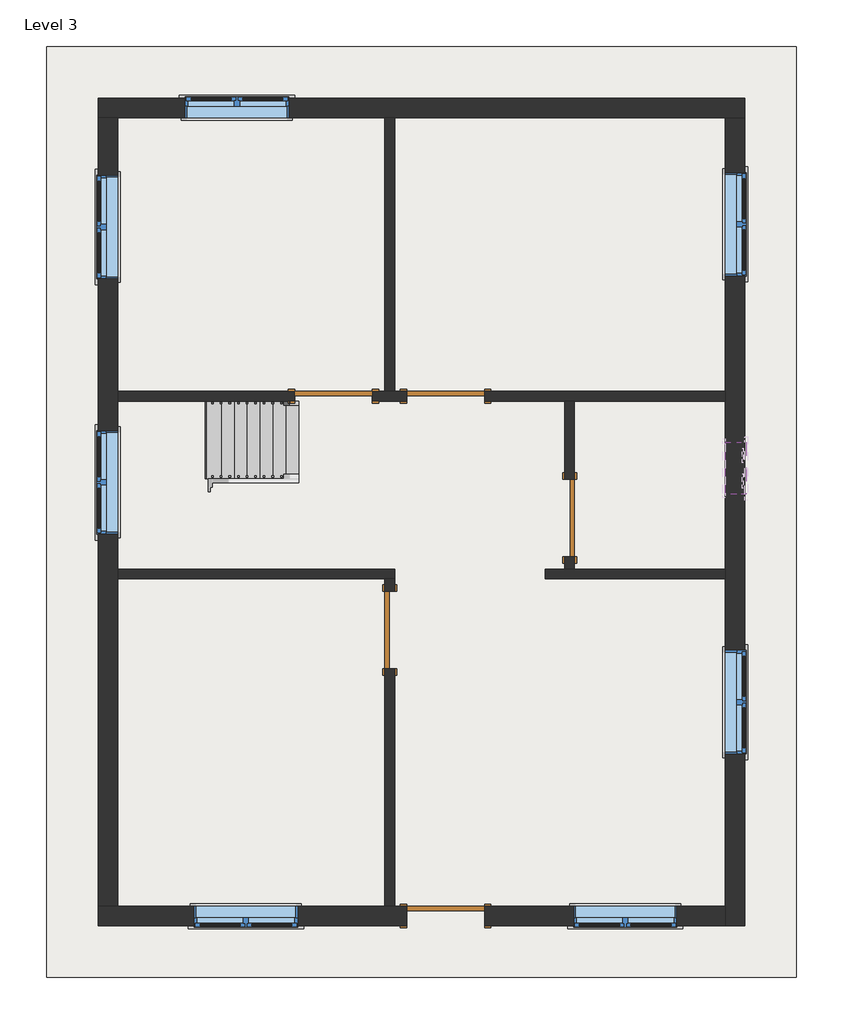
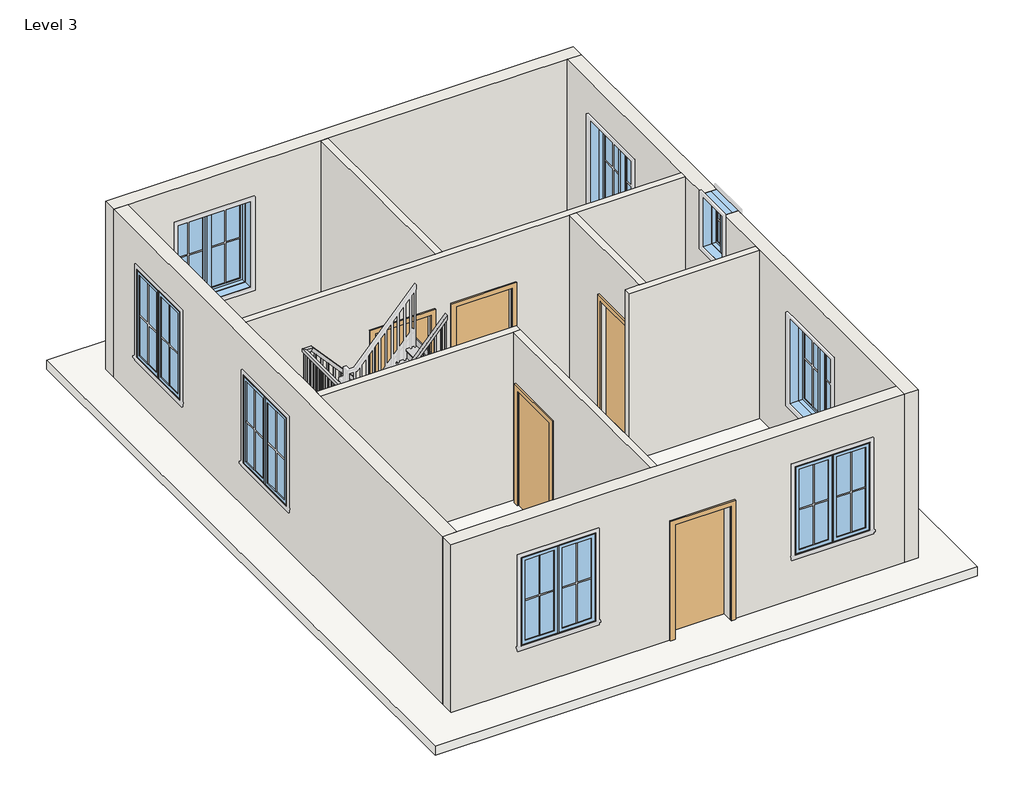
# One storey, part 1 of 2: 10 walls, 8 windows, 5 doors, 1 railing, 1 roof, 1 stair flight.
"""IFC4 building model written with IfcOpenShell, lengths in millimetres."""

from ifc_helpers import new_model, si_unit, frame, origin, place, context, project, spatial, polyline, outline, extrude, faceted_brep, transform, mapped, element, save
from components import door_e5f9f3c4, door_305aa2a5, door_a90ba1ad, stair_flight_173d3475, window_c417fced, window_8377141f

model = new_model("IFC4")

# Units and contexts
model_context = context("Model", 3, world=origin())
ifc_project = project(units=[si_unit("LENGTHUNIT", "METRE", prefix="MILLI")], contexts=[model_context])

# Site, building, storey
site = spatial("IfcSite", under=ifc_project)
building = spatial("IfcBuilding", under=site)
storey = spatial("IfcBuildingStorey", under=building, Name="Level 3", Elevation=6096.0)

# Doors
placement = place(None, origin())
door_shape = door_e5f9f3c4(model_context)
element("IfcDoor", 1, ObjectType="Single-Flush : 36\" x 84\"", at=placement, inside=storey, context=model_context, shape_type="MappedRepresentation", body=[
    mapped(door_shape, transform((4044.95, 10966.45, 6096.0), x_axis=(1.0, 0.0, 0.0), y_axis=(0.0, 1.0, 0.0), z_axis=(0.0, 0.0, 1.0))),
])
element("IfcDoor", 2, ObjectType="Single-Flush : 36\" x 84\"", at=placement, inside=storey, context=model_context, shape_type="MappedRepresentation", body=[
    mapped(door_shape, transform((4705.35, 8210.55, 6096.0), x_axis=(0.0, 1.0, 0.0), y_axis=(-1.0, 0.0, 0.0), z_axis=(0.0, 0.0, 1.0))),
])
element("IfcDoor", 3, ObjectType="Single-Flush : 36\" x 84\"", at=placement, inside=storey, context=model_context, shape_type="MappedRepresentation", body=[
    mapped(door_shape, transform((6826.25, 9531.35, 6096.0), x_axis=(0.0, -1.0, 0.0), y_axis=(1.0, 0.0, 0.0), z_axis=(0.0, 0.0, 1.0))),
])
door_2_shape = door_305aa2a5(model_context)
element("IfcDoor", 4, ObjectType="Single-Flush : 36\" x 84\"", at=placement, inside=storey, context=model_context, shape_type="MappedRepresentation", body=[
    mapped(door_2_shape, transform((5365.75, 10966.45, 6096.0), x_axis=(-1.0, 0.0, 0.0), y_axis=(0.0, -1.0, 0.0), z_axis=(0.0, 0.0, 1.0))),
])
door_3_shape = door_a90ba1ad(model_context)
element("IfcDoor", 5, ObjectType="Single-Flush : 36\" x 84\"", at=placement, inside=storey, context=model_context, shape_type="MappedRepresentation", body=[
    mapped(door_3_shape, transform((5365.75, 4838.7, 6096.0), x_axis=(-1.0, 0.0, 0.0), y_axis=(0.0, -1.0, 0.0), z_axis=(0.0, 0.0, 1.0))),
])

# Railing
element("IfcRailing", 6, ObjectType="Handrail - Rectangular", at=placement, inside=storey, context=model_context, shape_type="SolidModel", body=[
    faceted_brep([(3632.2, 10858.5, 7179.7333333), (3632.2, 10858.5, 7103.7950998), (3632.2, 10909.3, 7103.7950998), (3632.2, 10909.3, 7179.7333333), (2565.4, 10858.5, 8365.0666667), (2542.7755898, 10858.5, 8314.2666667), (2542.7755898, 10909.3, 8314.2666667), (2565.4, 10909.3, 8365.0666667), (2463.8, 10858.5, 8365.0666667), (2463.8, 10858.5, 8314.2666667), (2413.0, 10909.3, 8314.2666667), (2413.0, 10909.3, 8365.0666667), (2463.8, 9055.1, 8365.0666667), (2463.8, 9004.3, 8314.2666667), (2413.0, 9004.3, 8314.2666667), (2413.0, 9055.1, 8365.0666667), (2463.8, 9055.1, 8506.1777778), (2463.8, 9004.3, 8455.3777778), (2413.0, 9004.3, 8455.3777778), (2413.0, 9055.1, 8506.1777778), (2463.8, 8978.9, 8506.1777778), (2463.8, 8978.9, 8455.3777778), (2413.0, 8928.1, 8455.3777778), (2413.0, 8928.1, 8506.1777778), (2540.0, 8978.9, 8506.1777778), (2562.6244102, 8978.9, 8455.3777778), (2562.6244102, 8928.1, 8455.3777778), (2540.0, 8928.1, 8506.1777778), (3632.2, 8978.9, 9719.7333333), (3632.2, 8928.1, 9719.7333333), (3632.2, 8928.1, 9643.7950998), (3632.2, 8978.9, 9643.7950998)], [[[0, 1, 2, 3]], [[1, 0, 4, 5]], [[2, 1, 5, 6]], [[3, 2, 6, 7]], [[0, 3, 7, 4]], [[5, 4, 8, 9]], [[6, 5, 9, 10]], [[7, 6, 10, 11]], [[4, 7, 11, 8]], [[9, 8, 12, 13]], [[10, 9, 13, 14]], [[11, 10, 14, 15]], [[8, 11, 15, 12]], [[13, 12, 16, 17]], [[14, 13, 17, 18]], [[15, 14, 18, 19]], [[12, 15, 19, 16]], [[17, 16, 20, 21]], [[18, 17, 21, 22]], [[19, 18, 22, 23]], [[16, 19, 23, 20]], [[21, 20, 24, 25]], [[22, 21, 25, 26]], [[23, 22, 26, 27]], [[20, 23, 27, 24]], [[28, 29, 30, 31]], [[25, 24, 28, 31]], [[26, 25, 31, 30]], [[27, 26, 30, 29]], [[24, 27, 29, 28]]]),
    extrude(outline(polyline([(9569.7117665, 3565.525), (9548.5450998, 3546.475), (8636.0, 3546.475), (8636.0, 3565.525), (9569.7117665, 3565.525)])), frame((0.0, 8943.975, 0.0), z_axis=(0.0, 1.0, 0.0), x_axis=(0.0, 0.0, 1.0)), (0.0, 0.0, 1.0), 19.05),
    extrude(outline(polyline([(9456.8228776, 3463.925), (9435.6562109, 3444.875), (8466.6666667, 3444.875), (8466.6666667, 3463.925), (9456.8228776, 3463.925)])), frame((0.0, 8943.975, 0.0), z_axis=(0.0, 1.0, 0.0), x_axis=(0.0, 0.0, 1.0)), (0.0, 0.0, 1.0), 19.05),
    extrude(outline(polyline([(9343.9339887, 3362.325), (9322.767322, 3343.275), (8466.6666667, 3343.275), (8466.6666667, 3362.325), (9343.9339887, 3362.325)])), frame((0.0, 8943.975, 0.0), z_axis=(0.0, 1.0, 0.0), x_axis=(0.0, 0.0, 1.0)), (0.0, 0.0, 1.0), 19.05),
    extrude(outline(polyline([(9231.0450998, 3260.725), (9209.8784332, 3241.675), (8297.3333333, 3241.675), (8297.3333333, 3260.725), (9231.0450998, 3260.725)])), frame((0.0, 8943.975, 0.0), z_axis=(0.0, 1.0, 0.0), x_axis=(0.0, 0.0, 1.0)), (0.0, 0.0, 1.0), 19.05),
    extrude(outline(polyline([(9118.1562109, 3159.125), (9096.9895443, 3140.075), (8128.0, 3140.075), (8128.0, 3159.125), (9118.1562109, 3159.125)])), frame((0.0, 8943.975, 0.0), z_axis=(0.0, 1.0, 0.0), x_axis=(0.0, 0.0, 1.0)), (0.0, 0.0, 1.0), 19.05),
    extrude(outline(polyline([(9005.267322, 3057.525), (8984.1006554, 3038.475), (8128.0, 3038.475), (8128.0, 3057.525), (9005.267322, 3057.525)])), frame((0.0, 8943.975, 0.0), z_axis=(0.0, 1.0, 0.0), x_axis=(0.0, 0.0, 1.0)), (0.0, 0.0, 1.0), 19.05),
    extrude(outline(polyline([(8892.3784332, 2955.925), (8871.2117665, 2936.875), (7958.6666667, 2936.875), (7958.6666667, 2955.925), (8892.3784332, 2955.925)])), frame((0.0, 8943.975, 0.0), z_axis=(0.0, 1.0, 0.0), x_axis=(0.0, 0.0, 1.0)), (0.0, 0.0, 1.0), 19.05),
    extrude(outline(polyline([(8779.4895443, 2854.325), (8758.3228776, 2835.275), (7789.3333333, 2835.275), (7789.3333333, 2854.325), (8779.4895443, 2854.325)])), frame((0.0, 8943.975, 0.0), z_axis=(0.0, 1.0, 0.0), x_axis=(0.0, 0.0, 1.0)), (0.0, 0.0, 1.0), 19.05),
    extrude(outline(polyline([(8666.6006554, 2752.725), (8645.4339887, 2733.675), (7789.3333333, 2733.675), (7789.3333333, 2752.725), (8666.6006554, 2752.725)])), frame((0.0, 8943.975, 0.0), z_axis=(0.0, 1.0, 0.0), x_axis=(0.0, 0.0, 1.0)), (0.0, 0.0, 1.0), 19.05),
    extrude(outline(polyline([(8553.7117665, 2651.125), (8532.5450998, 2632.075), (7620.0, 2632.075), (7620.0, 2651.125), (8553.7117665, 2651.125)])), frame((0.0, 8943.975, 0.0), z_axis=(0.0, 1.0, 0.0), x_axis=(0.0, 0.0, 1.0)), (0.0, 0.0, 1.0), 19.05),
    extrude(outline(polyline([(8440.8228776, 2549.525), (8419.6562109, 2530.475), (7450.6666667, 2530.475), (7450.6666667, 2549.525), (8440.8228776, 2549.525)])), frame((0.0, 8943.975, 0.0), z_axis=(0.0, 1.0, 0.0), x_axis=(0.0, 0.0, 1.0)), (0.0, 0.0, 1.0), 19.05),
    extrude(outline(polyline([(2428.875, 9064.625), (2447.925, 9064.625), (2447.925, 9045.575), (2428.875, 9045.575), (2428.875, 9064.625)])), frame((0.0, 0.0, 7450.6666667), z_axis=(0.0, 0.0, 1.0), x_axis=(1.0, 0.0, 0.0)), (0.0, 0.0, 1.0), 863.6),
    extrude(outline(polyline([(2428.875, 9166.225), (2447.925, 9166.225), (2447.925, 9147.175), (2428.875, 9147.175), (2428.875, 9166.225)])), frame((0.0, 0.0, 7450.6666667), z_axis=(0.0, 0.0, 1.0), x_axis=(1.0, 0.0, 0.0)), (0.0, 0.0, 1.0), 863.6),
    extrude(outline(polyline([(2428.875, 9267.825), (2447.925, 9267.825), (2447.925, 9248.775), (2428.875, 9248.775), (2428.875, 9267.825)])), frame((0.0, 0.0, 7450.6666667), z_axis=(0.0, 0.0, 1.0), x_axis=(1.0, 0.0, 0.0)), (0.0, 0.0, 1.0), 863.6),
    extrude(outline(polyline([(2428.875, 9369.425), (2447.925, 9369.425), (2447.925, 9350.375), (2428.875, 9350.375), (2428.875, 9369.425)])), frame((0.0, 0.0, 7450.6666667), z_axis=(0.0, 0.0, 1.0), x_axis=(1.0, 0.0, 0.0)), (0.0, 0.0, 1.0), 863.6),
    extrude(outline(polyline([(2428.875, 9471.025), (2447.925, 9471.025), (2447.925, 9451.975), (2428.875, 9451.975), (2428.875, 9471.025)])), frame((0.0, 0.0, 7450.6666667), z_axis=(0.0, 0.0, 1.0), x_axis=(1.0, 0.0, 0.0)), (0.0, 0.0, 1.0), 863.6),
    extrude(outline(polyline([(2428.875, 9572.625), (2447.925, 9572.625), (2447.925, 9553.575), (2428.875, 9553.575), (2428.875, 9572.625)])), frame((0.0, 0.0, 7450.6666667), z_axis=(0.0, 0.0, 1.0), x_axis=(1.0, 0.0, 0.0)), (0.0, 0.0, 1.0), 863.6),
    extrude(outline(polyline([(2428.875, 9674.225), (2447.925, 9674.225), (2447.925, 9655.175), (2428.875, 9655.175), (2428.875, 9674.225)])), frame((0.0, 0.0, 7450.6666667), z_axis=(0.0, 0.0, 1.0), x_axis=(1.0, 0.0, 0.0)), (0.0, 0.0, 1.0), 863.6),
    extrude(outline(polyline([(2428.875, 9775.825), (2447.925, 9775.825), (2447.925, 9756.775), (2428.875, 9756.775), (2428.875, 9775.825)])), frame((0.0, 0.0, 7450.6666667), z_axis=(0.0, 0.0, 1.0), x_axis=(1.0, 0.0, 0.0)), (0.0, 0.0, 1.0), 863.6),
    extrude(outline(polyline([(2428.875, 9877.425), (2447.925, 9877.425), (2447.925, 9858.375), (2428.875, 9858.375), (2428.875, 9877.425)])), frame((0.0, 0.0, 7450.6666667), z_axis=(0.0, 0.0, 1.0), x_axis=(1.0, 0.0, 0.0)), (0.0, 0.0, 1.0), 863.6),
    extrude(outline(polyline([(2428.875, 9979.025), (2447.925, 9979.025), (2447.925, 9959.975), (2428.875, 9959.975), (2428.875, 9979.025)])), frame((0.0, 0.0, 7450.6666667), z_axis=(0.0, 0.0, 1.0), x_axis=(1.0, 0.0, 0.0)), (0.0, 0.0, 1.0), 863.6),
    extrude(outline(polyline([(2428.875, 10080.625), (2447.925, 10080.625), (2447.925, 10061.575), (2428.875, 10061.575), (2428.875, 10080.625)])), frame((0.0, 0.0, 7450.6666667), z_axis=(0.0, 0.0, 1.0), x_axis=(1.0, 0.0, 0.0)), (0.0, 0.0, 1.0), 863.6),
    extrude(outline(polyline([(2428.875, 10182.225), (2447.925, 10182.225), (2447.925, 10163.175), (2428.875, 10163.175), (2428.875, 10182.225)])), frame((0.0, 0.0, 7450.6666667), z_axis=(0.0, 0.0, 1.0), x_axis=(1.0, 0.0, 0.0)), (0.0, 0.0, 1.0), 863.6),
    extrude(outline(polyline([(2428.875, 10283.825), (2447.925, 10283.825), (2447.925, 10264.775), (2428.875, 10264.775), (2428.875, 10283.825)])), frame((0.0, 0.0, 7450.6666667), z_axis=(0.0, 0.0, 1.0), x_axis=(1.0, 0.0, 0.0)), (0.0, 0.0, 1.0), 863.6),
    extrude(outline(polyline([(2428.875, 10385.425), (2447.925, 10385.425), (2447.925, 10366.375), (2428.875, 10366.375), (2428.875, 10385.425)])), frame((0.0, 0.0, 7450.6666667), z_axis=(0.0, 0.0, 1.0), x_axis=(1.0, 0.0, 0.0)), (0.0, 0.0, 1.0), 863.6),
    extrude(outline(polyline([(2428.875, 10487.025), (2447.925, 10487.025), (2447.925, 10467.975), (2428.875, 10467.975), (2428.875, 10487.025)])), frame((0.0, 0.0, 7450.6666667), z_axis=(0.0, 0.0, 1.0), x_axis=(1.0, 0.0, 0.0)), (0.0, 0.0, 1.0), 863.6),
    extrude(outline(polyline([(2428.875, 10588.625), (2447.925, 10588.625), (2447.925, 10569.575), (2428.875, 10569.575), (2428.875, 10588.625)])), frame((0.0, 0.0, 7450.6666667), z_axis=(0.0, 0.0, 1.0), x_axis=(1.0, 0.0, 0.0)), (0.0, 0.0, 1.0), 863.6),
    extrude(outline(polyline([(2428.875, 10690.225), (2447.925, 10690.225), (2447.925, 10671.175), (2428.875, 10671.175), (2428.875, 10690.225)])), frame((0.0, 0.0, 7450.6666667), z_axis=(0.0, 0.0, 1.0), x_axis=(1.0, 0.0, 0.0)), (0.0, 0.0, 1.0), 863.6),
    extrude(outline(polyline([(2428.875, 10791.825), (2447.925, 10791.825), (2447.925, 10772.775), (2428.875, 10772.775), (2428.875, 10791.825)])), frame((0.0, 0.0, 7450.6666667), z_axis=(0.0, 0.0, 1.0), x_axis=(1.0, 0.0, 0.0)), (0.0, 0.0, 1.0), 863.6),
    extrude(outline(polyline([(2524.125, 10893.425), (2524.125, 10874.375), (2505.075, 10874.375), (2505.075, 10893.425), (2524.125, 10893.425)])), frame((0.0, 0.0, 7450.6666667), z_axis=(0.0, 0.0, 1.0), x_axis=(1.0, 0.0, 0.0)), (0.0, 0.0, 1.0), 863.6),
    extrude(outline(polyline([(8222.1006554, 2625.725), (8243.267322, 2606.675), (7281.3333333, 2606.675), (7281.3333333, 2625.725), (8222.1006554, 2625.725)])), frame((0.0, 10874.375, 0.0), z_axis=(0.0, 1.0, 0.0), x_axis=(0.0, 0.0, 1.0)), (0.0, 0.0, 1.0), 19.05),
    extrude(outline(polyline([(8109.2117665, 2727.325), (8130.3784332, 2708.275), (7281.3333333, 2708.275), (7281.3333333, 2727.325), (8109.2117665, 2727.325)])), frame((0.0, 10874.375, 0.0), z_axis=(0.0, 1.0, 0.0), x_axis=(0.0, 0.0, 1.0)), (0.0, 0.0, 1.0), 19.05),
    extrude(outline(polyline([(7996.3228776, 2828.925), (8017.4895443, 2809.875), (7112.0, 2809.875), (7112.0, 2828.925), (7996.3228776, 2828.925)])), frame((0.0, 10874.375, 0.0), z_axis=(0.0, 1.0, 0.0), x_axis=(0.0, 0.0, 1.0)), (0.0, 0.0, 1.0), 19.05),
    extrude(outline(polyline([(7883.4339887, 2930.525), (7904.6006554, 2911.475), (6942.6666667, 2911.475), (6942.6666667, 2930.525), (7883.4339887, 2930.525)])), frame((0.0, 10874.375, 0.0), z_axis=(0.0, 1.0, 0.0), x_axis=(0.0, 0.0, 1.0)), (0.0, 0.0, 1.0), 19.05),
    extrude(outline(polyline([(7770.5450998, 3032.125), (7791.7117665, 3013.075), (6942.6666667, 3013.075), (6942.6666667, 3032.125), (7770.5450998, 3032.125)])), frame((0.0, 10874.375, 0.0), z_axis=(0.0, 1.0, 0.0), x_axis=(0.0, 0.0, 1.0)), (0.0, 0.0, 1.0), 19.05),
    extrude(outline(polyline([(7657.6562109, 3133.725), (7678.8228776, 3114.675), (6773.3333333, 3114.675), (6773.3333333, 3133.725), (7657.6562109, 3133.725)])), frame((0.0, 10874.375, 0.0), z_axis=(0.0, 1.0, 0.0), x_axis=(0.0, 0.0, 1.0)), (0.0, 0.0, 1.0), 19.05),
    extrude(outline(polyline([(7544.767322, 3235.325), (7565.9339887, 3216.275), (6604.0, 3216.275), (6604.0, 3235.325), (7544.767322, 3235.325)])), frame((0.0, 10874.375, 0.0), z_axis=(0.0, 1.0, 0.0), x_axis=(0.0, 0.0, 1.0)), (0.0, 0.0, 1.0), 19.05),
    extrude(outline(polyline([(7431.8784332, 3336.925), (7453.0450998, 3317.875), (6604.0, 3317.875), (6604.0, 3336.925), (7431.8784332, 3336.925)])), frame((0.0, 10874.375, 0.0), z_axis=(0.0, 1.0, 0.0), x_axis=(0.0, 0.0, 1.0)), (0.0, 0.0, 1.0), 19.05),
    extrude(outline(polyline([(7318.9895443, 3438.525), (7340.1562109, 3419.475), (6434.6666667, 3419.475), (6434.6666667, 3438.525), (7318.9895443, 3438.525)])), frame((0.0, 10874.375, 0.0), z_axis=(0.0, 1.0, 0.0), x_axis=(0.0, 0.0, 1.0)), (0.0, 0.0, 1.0), 19.05),
    extrude(outline(polyline([(7206.1006554, 3540.125), (7227.267322, 3521.075), (6265.3333333, 3521.075), (6265.3333333, 3540.125), (7206.1006554, 3540.125)])), frame((0.0, 10874.375, 0.0), z_axis=(0.0, 1.0, 0.0), x_axis=(0.0, 0.0, 1.0)), (0.0, 0.0, 1.0), 19.05),
    extrude(outline(polyline([(2428.875, 8963.025), (2447.925, 8963.025), (2447.925, 8943.975), (2428.875, 8943.975), (2428.875, 8963.025)])), frame((0.0, 0.0, 7450.6666667), z_axis=(0.0, 0.0, 1.0), x_axis=(1.0, 0.0, 0.0)), (0.0, 0.0, 1.0), 1004.7111111),
    extrude(outline(polyline([(2447.925, 10893.425), (2447.925, 10874.375), (2428.875, 10874.375), (2428.875, 10893.425), (2447.925, 10893.425)])), frame((0.0, 0.0, 7450.6666667), z_axis=(0.0, 0.0, 1.0), x_axis=(1.0, 0.0, 0.0)), (0.0, 0.0, 1.0), 863.6),
    extrude(outline(polyline([(9643.7950998, 3632.2), (9622.6284332, 3613.15), (8636.0, 3613.15), (8636.0, 3632.2), (9643.7950998, 3632.2)])), frame((0.0, 8943.975, 0.0), z_axis=(0.0, 1.0, 0.0), x_axis=(0.0, 0.0, 1.0)), (0.0, 0.0, 1.0), 19.05),
    extrude(outline(polyline([(7103.7950998, 3632.2), (7124.9617665, 3613.15), (6265.3333333, 3613.15), (6265.3333333, 3632.2), (7103.7950998, 3632.2)])), frame((0.0, 10874.375, 0.0), z_axis=(0.0, 1.0, 0.0), x_axis=(0.0, 0.0, 1.0)), (0.0, 0.0, 1.0), 19.05),
])

# Roof
element("IfcRoof", 7, ObjectType="Generic - 12\"", at=placement, inside=storey, context=model_context, shape_type="SweptSolid", body=[
    extrude(outline(polyline([(660.4, 15087.6), (9499.6, 15087.6), (9499.6, 4114.8), (660.4, 4114.8), (660.4, 15087.6)])), frame((0.0, 0.0, 6096.0), z_axis=(0.0, 0.0, 1.0), x_axis=(1.0, 0.0, 0.0)), (0.0, 0.0, 1.0), 152.4),
])

# Stair flight
stair_flight_shape = stair_flight_173d3475(model_context)
element("IfcStairFlight", 8, ObjectType="2\" Tread 1\" Nosing 1/4\" Riser", at=placement, inside=storey, context=model_context, shape_type="MappedRepresentation", body=[
    mapped(stair_flight_shape, transform((0.0, 0.0, 0.0), x_axis=(1.0, 0.0, 0.0), y_axis=(0.0, 1.0, 0.0), z_axis=(0.0, 0.0, 1.0))),
])

# Walls
element("IfcWall", 9, ObjectType="Generic - 5\"", at=placement, inside=storey, context=model_context, shape_type="SweptSolid", body=[
    extrude(outline(polyline([(4648.2, 11023.6), (4648.2, 14249.4), (4762.5, 14249.4), (4762.5, 11023.6), (4648.2, 11023.6)])), frame((0.0, 0.0, 6096.0), z_axis=(0.0, 0.0, 1.0), x_axis=(1.0, 0.0, 0.0)), (0.0, 0.0, 1.0), 3048.0),
])
element("IfcWall", 10, ObjectType="Generic - 5\"", at=placement, inside=storey, context=model_context, shape_type="Brep", body=[
    faceted_brep([(4502.15, 10909.3, 6096.0), (4908.55, 10909.3, 6096.0), (4908.55, 10909.3, 8229.6), (5822.95, 10909.3, 8229.6), (5822.95, 10909.3, 6096.0), (6769.1, 10909.3, 6096.0), (6883.4, 10909.3, 6096.0), (8661.4, 10909.3, 6096.0), (8661.4, 10909.3, 9144.0), (6883.4, 10909.3, 9144.0), (6769.1, 10909.3, 9144.0), (1498.6, 10909.3, 9144.0), (1498.6, 10909.3, 6096.0), (3587.75, 10909.3, 6096.0), (3587.75, 10909.3, 8229.6), (4502.15, 10909.3, 8229.6), (4908.55, 11023.6, 8229.6), (4908.55, 11023.6, 6096.0), (4762.5, 11023.6, 6096.0), (4648.2, 11023.6, 6096.0), (4502.15, 11023.6, 6096.0), (4502.15, 11023.6, 8229.6), (3587.75, 11023.6, 8229.6), (3587.75, 11023.6, 6096.0), (1498.6, 11023.6, 6096.0), (1498.6, 11023.6, 9144.0), (4648.2, 11023.6, 9144.0), (4762.5, 11023.6, 9144.0), (8661.4, 11023.6, 9144.0), (8661.4, 11023.6, 6096.0), (5822.95, 11023.6, 6096.0), (5822.95, 11023.6, 8229.6)], [[[0, 1, 2, 3, 4, 5, 6, 7, 8, 9, 10, 11, 12, 13, 14, 15]], [[16, 17, 18, 19, 20, 21, 22, 23, 24, 25, 26, 27, 28, 29, 30, 31]], [[13, 12, 24, 23]], [[30, 29, 7, 6, 5, 4]], [[20, 19, 18, 17, 1, 0]], [[11, 10, 9, 8, 28, 27, 26, 25]], [[8, 7, 29, 28]], [[12, 11, 25, 24]], [[21, 20, 0, 15]], [[22, 21, 15, 14]], [[23, 22, 14, 13]], [[2, 1, 17, 16]], [[3, 2, 16, 31]], [[4, 3, 31, 30]]]),
])
element("IfcWall", 11, ObjectType="Generic - 5\"", at=placement, inside=storey, context=model_context, shape_type="SweptSolid", body=[
    extrude(outline(polyline([(9074.15, 8229.6), (9074.15, 6096.0), (8928.1, 6096.0), (8928.1, 9144.0), (10909.3, 9144.0), (10909.3, 6096.0), (9988.55, 6096.0), (9988.55, 8229.6), (9074.15, 8229.6)])), frame((6769.1, 0.0, 0.0), z_axis=(1.0, 0.0, 0.0), x_axis=(0.0, 1.0, 0.0)), (0.0, 0.0, 1.0), 114.3),
])
element("IfcWall", 12, ObjectType="Generic - 5\"", at=placement, inside=storey, context=model_context, shape_type="Brep", body=[
    faceted_brep([(1498.6, 8813.8, 6096.0), (4648.2, 8813.8, 6096.0), (4762.5, 8813.8, 6096.0), (4762.5, 8813.8, 9144.0), (4648.2, 8813.8, 9144.0), (1498.6, 8813.8, 9144.0), (1498.6, 8928.1, 6096.0), (1498.6, 8928.1, 9144.0), (4762.5, 8928.1, 9144.0), (4762.5, 8928.1, 6096.0)], [[[0, 1, 2, 3, 4, 5]], [[6, 7, 8, 9]], [[2, 1, 0, 6, 9]], [[5, 4, 3, 8, 7]], [[0, 5, 7, 6]], [[3, 2, 9, 8]]]),
])
element("IfcWall", 13, ObjectType="Generic - 5\"", at=placement, inside=storey, context=model_context, shape_type="SweptSolid", body=[
    extrude(outline(polyline([(8813.8, 6096.0), (8667.75, 6096.0), (8667.75, 8229.6), (7753.35, 8229.6), (7753.35, 6096.0), (4953.0, 6096.0), (4953.0, 9144.0), (8813.8, 9144.0), (8813.8, 6096.0)])), frame((4648.2, 0.0, 0.0), z_axis=(1.0, 0.0, 0.0), x_axis=(0.0, 1.0, 0.0)), (0.0, 0.0, 1.0), 114.3),
])
element("IfcWall", 14, ObjectType="Generic - 5\"", at=placement, inside=storey, context=model_context, shape_type="Brep", body=[
    faceted_brep([(6540.5050896, 8813.8, 6096.0), (8661.4, 8813.8, 6096.0), (8661.4, 8813.8, 9144.0), (6540.5050896, 8813.8, 9144.0), (6540.5050896, 8928.1, 6096.0), (6540.5050896, 8928.1, 9144.0), (6769.1, 8928.1, 9144.0), (6883.4, 8928.1, 9144.0), (8661.4, 8928.1, 9144.0), (8661.4, 8928.1, 6096.0), (6883.4, 8928.1, 6096.0), (6769.1, 8928.1, 6096.0)], [[[0, 1, 2, 3]], [[4, 5, 6, 7, 8, 9, 10, 11]], [[1, 0, 4, 11, 10, 9]], [[3, 2, 8, 7, 6, 5]], [[0, 3, 5, 4]], [[2, 1, 9, 8]]]),
])
element("IfcWall", 15, ObjectType="Generic - 8\"", at=placement, inside=storey, context=model_context, shape_type="Brep", body=[
    faceted_brep([(1270.0, 14249.4, 6096.0), (1498.6, 14249.4, 6096.0), (4648.2, 14249.4, 6096.0), (4762.5, 14249.4, 6096.0), (8661.4, 14249.4, 6096.0), (8890.0, 14249.4, 6096.0), (8890.0, 14249.4, 9144.0), (8661.4, 14249.4, 9144.0), (4762.5, 14249.4, 9144.0), (4648.2, 14249.4, 9144.0), (1498.6, 14249.4, 9144.0), (1270.0, 14249.4, 9144.0), (3514.725, 14249.4, 8534.4), (3514.725, 14249.4, 7010.4), (2295.525, 14249.4, 7010.4), (2295.525, 14249.4, 8534.4), (1270.0, 14478.0, 6096.0), (1270.0, 14478.0, 9144.0), (8890.0, 14478.0, 9144.0), (8890.0, 14478.0, 6096.0), (3514.725, 14478.0, 8534.4), (2295.525, 14478.0, 8534.4), (2295.525, 14478.0, 7010.4), (3514.725, 14478.0, 7010.4)], [[[0, 1, 2, 3, 4, 5, 6, 7, 8, 9, 10, 11], [12, 13, 14, 15]], [[16, 17, 18, 19], [20, 21, 22, 23]], [[5, 4, 3, 2, 1, 0, 16, 19]], [[11, 10, 9, 8, 7, 6, 18, 17]], [[6, 5, 19, 18]], [[0, 11, 17, 16]], [[13, 12, 20, 23]], [[14, 13, 23, 22]], [[15, 14, 22, 21]], [[12, 15, 21, 20]]]),
])
element("IfcWall", 16, ObjectType="Generic - 8\"", at=placement, inside=storey, context=model_context, shape_type="Brep", body=[
    faceted_brep([(8661.4, 14249.4, 6096.0), (8661.4, 11023.6, 6096.0), (8661.4, 10909.3, 6096.0), (8661.4, 8928.1, 6096.0), (8661.4, 8813.8, 6096.0), (8661.4, 4953.0, 6096.0), (8661.4, 4724.4, 6096.0), (8661.4, 4724.4, 9144.0), (8661.4, 4953.0, 9144.0), (8661.4, 8813.8, 9144.0), (8661.4, 8928.1, 9144.0), (8661.4, 9810.75, 9144.0), (8661.4, 9810.75, 8229.6), (8661.4, 10420.35, 8229.6), (8661.4, 10420.35, 9144.0), (8661.4, 10909.3, 9144.0), (8661.4, 11023.6, 9144.0), (8661.4, 14249.4, 9144.0), (8661.4, 6750.05, 8534.4), (8661.4, 6750.05, 7010.4), (8661.4, 7969.25, 7010.4), (8661.4, 7969.25, 8534.4), (8661.4, 12382.5, 8534.4), (8661.4, 12382.5, 7010.4), (8661.4, 13601.7, 7010.4), (8661.4, 13601.7, 8534.4), (8890.0, 4724.4, 6096.0), (8890.0, 14249.4, 6096.0), (8890.0, 14249.4, 9144.0), (8890.0, 10420.35, 9144.0), (8890.0, 10420.35, 8229.6), (8890.0, 9810.75, 8229.6), (8890.0, 9810.75, 9144.0), (8890.0, 4724.4, 9144.0), (8890.0, 6750.05, 7010.4), (8890.0, 6750.05, 8534.4), (8890.0, 7969.25, 8534.4), (8890.0, 7969.25, 7010.4), (8890.0, 12382.5, 7010.4), (8890.0, 12382.5, 8534.4), (8890.0, 13601.7, 8534.4), (8890.0, 13601.7, 7010.4)], [[[0, 1, 2, 3, 4, 5, 6, 7, 8, 9, 10, 11, 12, 13, 14, 15, 16, 17], [18, 19, 20, 21], [22, 23, 24, 25]], [[26, 27, 28, 29, 30, 31, 32, 33], [34, 35, 36, 37], [38, 39, 40, 41]], [[6, 5, 4, 3, 2, 1, 0, 27, 26]], [[28, 17, 16, 15, 14, 29]], [[7, 33, 32, 11, 10, 9, 8]], [[0, 17, 28, 27]], [[7, 6, 26, 33]], [[19, 18, 35, 34]], [[20, 19, 34, 37]], [[21, 20, 37, 36]], [[18, 21, 36, 35]], [[23, 22, 39, 38]], [[24, 23, 38, 41]], [[25, 24, 41, 40]], [[22, 25, 40, 39]], [[31, 12, 11, 32]], [[12, 31, 30, 13]], [[13, 30, 29, 14]]]),
])
element("IfcWall", 17, ObjectType="Generic - 8\"", at=placement, inside=storey, context=model_context, shape_type="Brep", body=[
    faceted_brep([(4908.55, 4953.0, 8229.6), (4908.55, 4953.0, 6096.0), (4762.5, 4953.0, 6096.0), (4648.2, 4953.0, 6096.0), (1498.6, 4953.0, 6096.0), (1270.0, 4953.0, 6096.0), (1270.0, 4953.0, 9144.0), (1498.6, 4953.0, 9144.0), (4648.2, 4953.0, 9144.0), (4762.5, 4953.0, 9144.0), (8661.4, 4953.0, 9144.0), (8661.4, 4953.0, 6096.0), (5822.95, 4953.0, 6096.0), (5822.95, 4953.0, 8229.6), (2400.3, 4953.0, 8534.4), (2400.3, 4953.0, 7010.4), (3619.5, 4953.0, 7010.4), (3619.5, 4953.0, 8534.4), (6872.2875, 4953.0, 8534.4), (6872.2875, 4953.0, 7010.4), (8091.4875, 4953.0, 7010.4), (8091.4875, 4953.0, 8534.4), (1270.0, 4724.4, 6096.0), (4908.55, 4724.4, 6096.0), (4908.55, 4724.4, 8229.6), (5822.95, 4724.4, 8229.6), (5822.95, 4724.4, 6096.0), (8661.4, 4724.4, 6096.0), (8661.4, 4724.4, 9144.0), (1270.0, 4724.4, 9144.0), (2400.3, 4724.4, 8534.4), (3619.5, 4724.4, 8534.4), (3619.5, 4724.4, 7010.4), (2400.3, 4724.4, 7010.4), (6872.2875, 4724.4, 8534.4), (8091.4875, 4724.4, 8534.4), (8091.4875, 4724.4, 7010.4), (6872.2875, 4724.4, 7010.4)], [[[0, 1, 2, 3, 4, 5, 6, 7, 8, 9, 10, 11, 12, 13], [14, 15, 16, 17], [18, 19, 20, 21]], [[22, 23, 24, 25, 26, 27, 28, 29], [30, 31, 32, 33], [34, 35, 36, 37]], [[12, 11, 27, 26]], [[5, 4, 3, 2, 1, 23, 22]], [[10, 9, 8, 7, 6, 29, 28]], [[11, 10, 28, 27]], [[6, 5, 22, 29]], [[24, 23, 1, 0]], [[25, 24, 0, 13]], [[26, 25, 13, 12]], [[15, 14, 30, 33]], [[16, 15, 33, 32]], [[17, 16, 32, 31]], [[14, 17, 31, 30]], [[19, 18, 34, 37]], [[20, 19, 37, 36]], [[21, 20, 36, 35]], [[18, 21, 35, 34]]]),
])
element("IfcWall", 18, ObjectType="Generic - 8\"", at=placement, inside=storey, context=model_context, shape_type="Brep", body=[
    faceted_brep([(1498.6, 4953.0, 6096.0), (1498.6, 8813.8, 6096.0), (1498.6, 8928.1, 6096.0), (1498.6, 10909.3, 6096.0), (1498.6, 11023.6, 6096.0), (1498.6, 14249.4, 6096.0), (1498.6, 14249.4, 9144.0), (1498.6, 11023.6, 9144.0), (1498.6, 10909.3, 9144.0), (1498.6, 8928.1, 9144.0), (1498.6, 8813.8, 9144.0), (1498.6, 4953.0, 9144.0), (1498.6, 13569.95, 8534.4), (1498.6, 13569.95, 7010.4), (1498.6, 12350.75, 7010.4), (1498.6, 12350.75, 8534.4), (1498.6, 10560.05, 8534.4), (1498.6, 10560.05, 7010.4), (1498.6, 9340.85, 7010.4), (1498.6, 9340.85, 8534.4), (1270.0, 14249.4, 6096.0), (1270.0, 4953.0, 6096.0), (1270.0, 4953.0, 9144.0), (1270.0, 14249.4, 9144.0), (1270.0, 13569.95, 7010.4), (1270.0, 13569.95, 8534.4), (1270.0, 12350.75, 8534.4), (1270.0, 12350.75, 7010.4), (1270.0, 10560.05, 7010.4), (1270.0, 10560.05, 8534.4), (1270.0, 9340.85, 8534.4), (1270.0, 9340.85, 7010.4)], [[[0, 1, 2, 3, 4, 5, 6, 7, 8, 9, 10, 11], [12, 13, 14, 15], [16, 17, 18, 19]], [[20, 21, 22, 23], [24, 25, 26, 27], [28, 29, 30, 31]], [[5, 4, 3, 2, 1, 0, 21, 20]], [[11, 10, 9, 8, 7, 6, 23, 22]], [[6, 5, 20, 23]], [[0, 11, 22, 21]], [[13, 12, 25, 24]], [[14, 13, 24, 27]], [[15, 14, 27, 26]], [[12, 15, 26, 25]], [[17, 16, 29, 28]], [[18, 17, 28, 31]], [[19, 18, 31, 30]], [[16, 19, 30, 29]]]),
])

# Windows
window_shape = window_c417fced(model_context)
element("IfcWindow", 19, ObjectType="Window-Casement-Double : 24\" x 36\"", at=placement, inside=storey, context=model_context, shape_type="MappedRepresentation", body=[
    mapped(window_shape, transform((8775.7, 10115.55, 7315.2), x_axis=(0.0, -1.0, 0.0), y_axis=(1.0, 0.0, 0.0), z_axis=(0.0, 0.0, 1.0))),
])
window_2_shape = window_8377141f(model_context)
element("IfcWindow", 20, ObjectType="Window-Casement-Double : 48\" x 60\"", at=placement, inside=storey, context=model_context, shape_type="MappedRepresentation", body=[
    mapped(window_2_shape, transform((7481.8875, 4838.7, 6096.0), x_axis=(-1.0, 0.0, 0.0), y_axis=(0.0, -1.0, 0.0), z_axis=(0.0, 0.0, 1.0))),
])
element("IfcWindow", 21, ObjectType="Window-Casement-Double : 48\" x 60\"", at=placement, inside=storey, context=model_context, shape_type="MappedRepresentation", body=[
    mapped(window_2_shape, transform((3009.9, 4838.7, 6096.0), x_axis=(-1.0, 0.0, 0.0), y_axis=(0.0, -1.0, 0.0), z_axis=(0.0, 0.0, 1.0))),
])
element("IfcWindow", 22, ObjectType="Window-Casement-Double : 48\" x 60\"", at=placement, inside=storey, context=model_context, shape_type="MappedRepresentation", body=[
    mapped(window_2_shape, transform((8775.7, 12992.1, 6096.0), x_axis=(0.0, -1.0, 0.0), y_axis=(1.0, 0.0, 0.0), z_axis=(0.0, 0.0, 1.0))),
])
element("IfcWindow", 23, ObjectType="Window-Casement-Double : 48\" x 60\"", at=placement, inside=storey, context=model_context, shape_type="MappedRepresentation", body=[
    mapped(window_2_shape, transform((8775.7, 7359.65, 6096.0), x_axis=(0.0, -1.0, 0.0), y_axis=(1.0, 0.0, 0.0), z_axis=(0.0, 0.0, 1.0))),
])
element("IfcWindow", 24, ObjectType="Window-Casement-Double : 48\" x 60\"", at=placement, inside=storey, context=model_context, shape_type="MappedRepresentation", body=[
    mapped(window_2_shape, transform((1384.3, 12960.35, 6096.0), x_axis=(0.0, 1.0, 0.0), y_axis=(-1.0, 0.0, 0.0), z_axis=(0.0, 0.0, 1.0))),
])
element("IfcWindow", 25, ObjectType="Window-Casement-Double : 48\" x 60\"", at=placement, inside=storey, context=model_context, shape_type="MappedRepresentation", body=[
    mapped(window_2_shape, transform((1384.3, 9950.45, 6096.0), x_axis=(0.0, 1.0, 0.0), y_axis=(-1.0, 0.0, 0.0), z_axis=(0.0, 0.0, 1.0))),
])
element("IfcWindow", 26, ObjectType="Window-Casement-Double : 48\" x 60\"", at=placement, inside=storey, context=model_context, shape_type="MappedRepresentation", body=[
    mapped(window_2_shape, transform((2905.125, 14363.7, 6096.0), x_axis=(1.0, 0.0, 0.0), y_axis=(0.0, 1.0, 0.0), z_axis=(0.0, 0.0, 1.0))),
])

save(model, "model.ifc")

# Revit data of these elements
# Type "Single-Flush : 36\" x 84\""
#   Type Mark = "1"
#   Construction Type Id = "MDOOR"
#   Assembly Code = "C1020"
#   Analytic Construction = "Metal"
#   Thickness = 0' - 2"
#   Heat Transfer Coefficient (U) = 0.651978 BTU/(h·ft²·°F)
#   Height = 7' - 0"
#   Trim Projection Ext = 0' - 1"
#   Trim Projection Int = 0' - 1"
#   Trim Width = 0' - 3"
#   Width = 3' - 0"
#   Define Thermal Properties by = 1
#   Define Thermal Properties by = 1
#   Door Material = Door - Panel
#   Frame Material = Door - Frame
#   Visual Light Transmittance = 0
#   Solar Heat Gain Coefficient = 0
#   Function = (empty or 0)
#   Wall Closure = (empty or 0)
# Type "Handrail - Rectangular"
#   Assembly Code = "C2010400"
#   built-in parameter 1008612 = 0.0416667 (stored number, unit not read)
#   built-in parameter 1008611 = 0.0416667 (stored number, unit not read)
#   built-in parameter 1008609 = 0.333333 (stored number, unit not read)
#   built-in parameter 1008604 = 0.166667 (stored number, unit not read)
#   built-in parameter 1008603 = 0.166667 (stored number, unit not read)
#   Railing Height = 3' - 0"
#   built-in parameter 1008630 = 2
#   built-in parameter 1008610 = 2
#   built-in parameter 1008618 = Baluster - Square : 3/4"
# Type "Generic - 12\""
#   Assembly Code = "B1020"
#   Layers, outside or top first: 0' - 6" no material (function 1)
# Type "Generic - 5\""
#   Assembly Code = "B2010"
#   Layers, outside or top first: 0' - 4 1/2" no material (function 1)
# Type "Generic - 8\""
#   Assembly Code = "B2010"
#   Layers, outside or top first: 0' - 9" "Parking Stripe" (function 1)
# Type "Window-Casement-Double : 24\" x 36\""
#   Type Mark = "14"
#   Fire Rating = "0.5h"
#   Assembly Code = "B2020100"
#   Analytic Construction = "Double glazing - domestic"
#   Frame Extension [instance default] = 0' - 0 1/4"
#   Window Inset [instance default] = 0' - 0"
#   Wall Thickness [instance default] = 0' - 6"
#   Interior Wall Closure [instance default] = 0' - 2 1/4"
#   Half Width = 1' - 0"
#   Visual Light Transmittance = 0.81
#   Thermal Resistance (R) = 1.8146 (h·ft²·°F)/BTU
#   Solar Heat Gain Coefficient = 0.76
#   Rough Width = 2' - 0 1/2"
#   Rough Height = 3' - 0 1/2"
#   Height = 3' - 0"
#   Heat Transfer Coefficient (U) = 0.5511 BTU/(h·ft²·°F)
#   Exterior Wall Closure [instance default] = 0' - 1 1/4"
#   Extension Jamb [instance default] = 0' - 2 1/4"
#   Default Sill Height = 3' - 0"
#   Width = 2' - 0"
#   Define Thermal Properties by = 0
#   Muntin Visibility = yes
#   Interior Trim Visibility [instance default] = yes
#   Exterior Trim Visibility [instance default] = yes
#   Extension Jamb Visibility [instance default] = yes
#   Interior Trim Material = Wood - Stained
#   Muntin Pattern = Muntin Pattern_2x2 : Muntin Pattern_2x2
#   Interior Trim = Trim-Window-Interior-Flat : Picture Frame
#   Interior Frame Material = Wood - Stained
#   Glass Panel Material = Glass
#   Exterior Trim Material = Clad - White
#   Exterior Trim = Trim-Window-Exterior-Flat : with Sill
#   Exterior Frame Material = Clad - White
#   Wall Closure = (empty or 0)
# Type "Window-Casement-Double : 48\" x 60\""
#   Type Mark = "17"
#   Fire Rating = "0.5h"
#   Assembly Code = "B2020100"
#   Analytic Construction = "Double glazing - domestic"
#   Frame Extension [instance default] = 0' - 0 1/4"
#   Window Inset [instance default] = 0' - 0"
#   Wall Thickness [instance default] = 0' - 6"
#   Interior Wall Closure [instance default] = 0' - 2 1/4"
#   Half Width = 2' - 0"
#   Visual Light Transmittance = 0.81
#   Thermal Resistance (R) = 1.8146 (h·ft²·°F)/BTU
#   Solar Heat Gain Coefficient = 0.76
#   Rough Width = 4' - 0 1/2"
#   Rough Height = 5' - 0 1/2"
#   Height = 5' - 0"
#   Heat Transfer Coefficient (U) = 0.5511 BTU/(h·ft²·°F)
#   Exterior Wall Closure [instance default] = 0' - 1 1/4"
#   Extension Jamb [instance default] = 0' - 2 1/4"
#   Default Sill Height = 3' - 0"
#   Width = 4' - 0"
#   Define Thermal Properties by = 0
#   Muntin Visibility = yes
#   Interior Trim Visibility [instance default] = yes
#   Exterior Trim Visibility [instance default] = yes
#   Extension Jamb Visibility [instance default] = yes
#   Interior Trim Material = Wood - Stained
#   Muntin Pattern = Muntin Pattern_2x2 : Muntin Pattern_2x2
#   Interior Trim = Trim-Window-Interior-Flat : Picture Frame
#   Interior Frame Material = Wood - Stained
#   Glass Panel Material = Glass
#   Exterior Trim Material = Clad - White
#   Exterior Trim = Trim-Window-Exterior-Flat : with Sill
#   Exterior Frame Material = Clad - White
#   Wall Closure = (empty or 0)
# Elements 1, 2, 3, 4, 5 (IfcDoor, "Single-Flush : 36\" x 84\"")
#   Phase Created = New Construction
#   Materials on its faces: "Door - Frame", "Door - Panel"
# Element 6 (IfcRailing, "Handrail - Rectangular")
#   Phase Created = New Construction
# Element 7 (IfcRoof, "Generic - 12\"")
#   built-in parameter 1001705 = 20.5 (stored number, unit not read)
#   built-in parameter 1001710 = 33615
#   Phase Created = New Construction
#   Materials on its faces: "Textile - Linen, Smooth", "Default Roof"
# Element 8 (IfcStairFlight, "2\" Tread 1\" Nosing 1/4\" Riser")
#   Phase Created = New Construction
# Elements 9, 10, 11, 12, 13, 14 (IfcWall, "Generic - 5\"")
#   Top Offset = 0' - 0"
#   Base Offset = 0' - 0"
#   wall height = 10' - 0"
#   Phase Created = New Construction
#   Base Constraint = Level 3
#   Top Constraint = Level 4
#   Materials on its faces: "Default Wall"
# Elements 15, 16, 17, 18 (IfcWall, "Generic - 8\"")
#   Top Offset = 0' - 0"
#   Base Offset = 0' - 0"
#   Unconnected Height = 10' - 0"
#   wall height = 10' - 0"
#   Phase Created = New Construction
#   Base Constraint = Level 3
#   Materials on its faces: "Parking Stripe", "Wood Planks"
# Element 19 (IfcWindow, "Window-Casement-Double : 24\" x 36\"")
#   Mark = "24"
#   Window Inset = 0' - 0"
#   Interior Wall Closure = 0' - 2 1/4"
#   Frame Extension = 0' - 0 1/4"
#   Exterior Wall Closure = 0' - 1 1/4"
#   Interior Trim Visibility = yes
#   Exterior Trim Visibility = yes
#   Phase Created = New Construction
#   Materials on its faces: "Wood - Stained", "Glass", "Clad - White"
# Element 20 (IfcWindow, "Window-Casement-Double : 48\" x 60\"")
#   Mark = "11"
#   Window Inset = 0' - 0"
#   Interior Wall Closure = 0' - 2 1/4"
#   Frame Extension = 0' - 0 1/4"
#   Exterior Wall Closure = 0' - 1 1/4"
#   Interior Trim Visibility = yes
#   Exterior Trim Visibility = yes
#   Phase Created = New Construction
#   Materials on its faces: "Wood - Stained", "Glass", "Clad - White"
# Element 21 (IfcWindow, "Window-Casement-Double : 48\" x 60\"")
#   Mark = "12"
#   Window Inset = 0' - 0"
#   Interior Wall Closure = 0' - 2 1/4"
#   Frame Extension = 0' - 0 1/4"
#   Exterior Wall Closure = 0' - 1 1/4"
#   Interior Trim Visibility = yes
#   Exterior Trim Visibility = yes
#   Phase Created = New Construction
#   Materials on its faces: "Wood - Stained", "Glass", "Clad - White"
# Element 22 (IfcWindow, "Window-Casement-Double : 48\" x 60\"")
#   Mark = "22"
#   Window Inset = 0' - 0"
#   Interior Wall Closure = 0' - 2 1/4"
#   Frame Extension = 0' - 0 1/4"
#   Exterior Wall Closure = 0' - 1 1/4"
#   Interior Trim Visibility = yes
#   Exterior Trim Visibility = yes
#   Phase Created = New Construction
#   Materials on its faces: "Wood - Stained", "Glass", "Clad - White"
# Element 23 (IfcWindow, "Window-Casement-Double : 48\" x 60\"")
#   Mark = "23"
#   Window Inset = 0' - 0"
#   Interior Wall Closure = 0' - 2 1/4"
#   Frame Extension = 0' - 0 1/4"
#   Exterior Wall Closure = 0' - 1 1/4"
#   Interior Trim Visibility = yes
#   Exterior Trim Visibility = yes
#   Phase Created = New Construction
#   Materials on its faces: "Wood - Stained", "Glass", "Clad - White"
# Element 24 (IfcWindow, "Window-Casement-Double : 48\" x 60\"")
#   Mark = "35"
#   Window Inset = 0' - 0"
#   Interior Wall Closure = 0' - 2 1/4"
#   Frame Extension = 0' - 0 1/4"
#   Exterior Wall Closure = 0' - 1 1/4"
#   Interior Trim Visibility = yes
#   Exterior Trim Visibility = yes
#   Phase Created = New Construction
#   Materials on its faces: "Wood - Stained", "Glass", "Clad - White"
# Element 25 (IfcWindow, "Window-Casement-Double : 48\" x 60\"")
#   Mark = "39"
#   Window Inset = 0' - 0"
#   Interior Wall Closure = 0' - 2 1/4"
#   Frame Extension = 0' - 0 1/4"
#   Exterior Wall Closure = 0' - 1 1/4"
#   Interior Trim Visibility = yes
#   Exterior Trim Visibility = yes
#   Phase Created = New Construction
#   Materials on its faces: "Wood - Stained", "Glass", "Clad - White"
# Element 26 (IfcWindow, "Window-Casement-Double : 48\" x 60\"")
#   Mark = "49"
#   Window Inset = 0' - 0"
#   Interior Wall Closure = 0' - 2 1/4"
#   Frame Extension = 0' - 0 1/4"
#   Exterior Wall Closure = 0' - 1 1/4"
#   Interior Trim Visibility = yes
#   Exterior Trim Visibility = yes
#   Phase Created = New Construction
#   Materials on its faces: "Wood - Stained", "Glass", "Clad - White"
# Materials
#   "Door - Panel": class "Wood", colour RGB 210 159 95, transparency 0, Cost = 0
#   "Door - Frame": colour RGB 118 70 51, transparency 0, Cost = 0
#   "Parking Stripe": class "Paint", colour RGB 250 250 91, transparency 0, Cost = 0
#   "Wood - Stained": class "Wood", colour RGB 224 178 126, transparency 0, Cost = 0
#   "Glass": class "Glass", colour RGB 0 128 192, transparency 0.75, Description = "Soda Lime Glass", Cost = 0
#   "Clad - White": class "Wood", colour RGB 242 242 238, transparency 0, Cost = 0
#   "Textile - Linen, Smooth": colour RGB 249 239 230, transparency 0
#   "Default Roof": colour RGB 88 101 114, transparency 0, Cost = 0
#   "Default Wall": colour RGB 128 128 128, transparency 0, Cost = 0
#   "Wood Planks": class "Wood", colour RGB 193 160 115, transparency 0, Description = "Physical material.", Cost = 0
